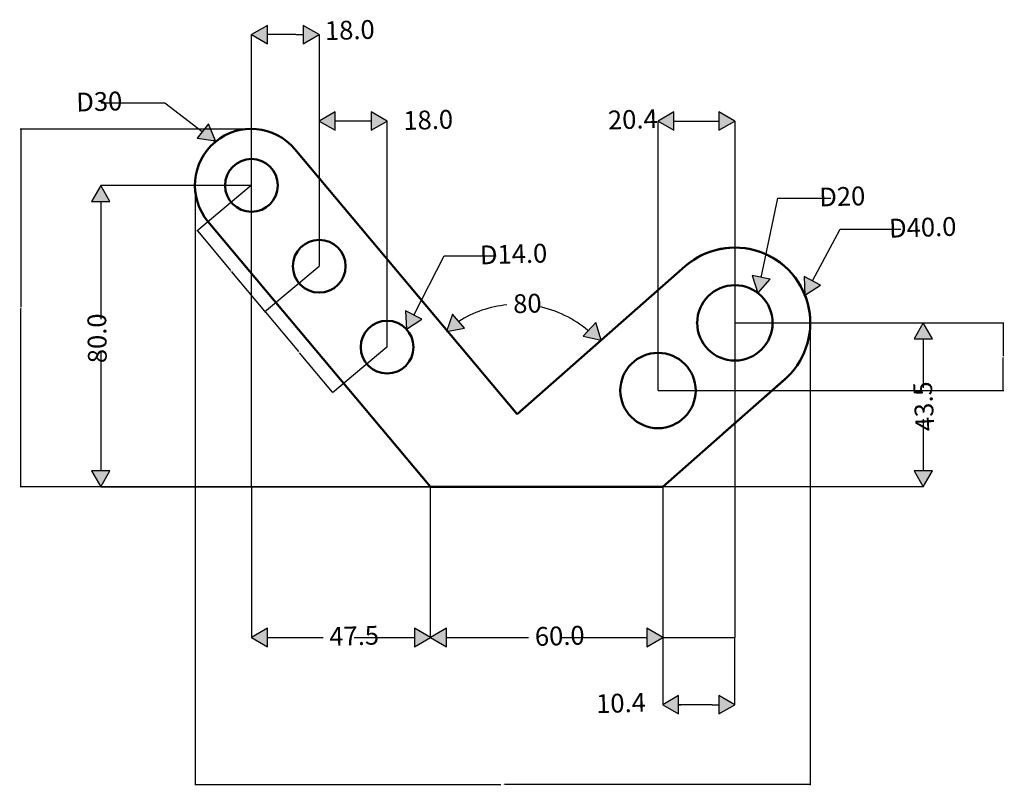
# Model space of a CAD drawing. Units: millimetres. Extents: x 651 to 912, y 1072 to 1275.
import ezdxf

# ---------------------------------------------------------------- set-up
doc = ezdxf.new("R2010")
doc.units = ezdxf.units.MM
for name, color, linetype, lineweight in [('M-CONS', 8, 'Continuous', 13), ('M-DIMS', 2, 'Continuous', 25), ('M-HATC', 2, 'Continuous', 18), ('M-OUTL', 7, 'Continuous', 50), ('M-TEXT', 7, 'Continuous', 25)]:
    doc.layers.add(name, color=color, linetype=linetype, lineweight=lineweight)
doc.styles.get("Standard").update_dxf_attribs({"font": 'arial.ttf'})
doc.dimstyles.get("Standard").update_dxf_attribs({"dimtxt": 0.18, "dimasz": 0.18, "dimexe": 0.18, "dimexo": 0.0625, "dimgap": 0.09, "dimtad": 0, "dimtih": 1, "dimtoh": 1, "dimdec": 4, "dimzin": 0, "dimdsep": 46, "dimtxsty": 'Standard', "dimcen": 0.09, "dimadec": 0, "dimazin": 0, "dimtfac": 1, "dimtdec": 4, "dimtofl": 0, "dimtmove": 0, "dimatfit": 3, "dimfxl": 1, "dimtolj": 1, "dimtzin": 0, "dimarcsym": 0})

# ---------------------------------------------------------------- blocks, each defined once
blk = doc.blocks.new('LINK-HOLE-D14')
blk.add_circle((7, 7), 7)
blk = doc.blocks.new('LINK-HOLE-D20')
blk.add_circle((10, 10), 10)
blk = doc.blocks.new('*D3')
at = {"layer": 'Defpoints', "color": 0, "transparency": 16777216}
for p in [(697.1, 1232.79), (860.34, 1194.98), (860.34, 1072.44)]:
    blk.add_point(p, dxfattribs=at)
at = {"layer": 'M-DIMS', "color": 0, "lineweight": -2, "transparency": 16777216}
for p, q in [((697.1, 1232.73), (697.1, 1072.26)), ((860.34, 1194.92), (860.34, 1072.26)), ((697.28, 1072.44), (778.26, 1072.44)), ((860.16, 1072.44), (779.17, 1072.44))]:
    blk.add_line(p, q, dxfattribs=at)
at = {"layer": 'M-DIMS', "color": 0, "transparency": 16777216}
for points in [[(697.28, 1072.47), (697.28, 1072.41), (697.1, 1072.44)], [(860.16, 1072.47), (860.16, 1072.41), (860.34, 1072.44)]]:
    blk.add_solid(points, dxfattribs=at)
at = {"layer": 'M-DIMS', "color": 0, "transparency": 16777216, "insert": (778.72, 1072.44), "char_height": 0.18, "attachment_point": 5}
blk.add_mtext('\\A1;163.24', dxfattribs=at)
blk = doc.blocks.new('*D4')
at = {"layer": 'Defpoints', "color": 0, "transparency": 16777216}
for p in [(713.35, 1246.42), (650.84, 1151.48), (759.54, 1151.48)]:
    blk.add_point(p, dxfattribs=at)
at = {"layer": 'M-DIMS', "color": 0, "lineweight": -2, "transparency": 16777216}
for p, q in [((713.29, 1246.42), (650.66, 1246.42)), ((650.84, 1246.24), (650.84, 1199.13)), ((650.84, 1151.66), (650.84, 1198.77)), ((759.48, 1151.48), (650.66, 1151.48))]:
    blk.add_line(p, q, dxfattribs=at)
at = {"layer": 'M-DIMS', "color": 0, "transparency": 16777216}
for points in [[(650.81, 1246.24), (650.87, 1246.24), (650.84, 1246.42)], [(650.81, 1151.66), (650.87, 1151.66), (650.84, 1151.48)]]:
    blk.add_solid(points, dxfattribs=at)
at = {"layer": 'M-DIMS', "color": 0, "transparency": 16777216, "insert": (650.84, 1198.95), "char_height": 0.18, "attachment_point": 5}
blk.add_mtext('\\A1;94.94', dxfattribs=at)
blk = doc.blocks.new('*D5')
at = {"layer": 'Defpoints', "color": 0, "transparency": 16777216}
for p in [(712.04, 1231.48), (697.67, 1219.43), (730.04, 1210.01)]:
    blk.add_point(p, dxfattribs=at)
at = {"layer": 'M-DIMS', "color": 0, "lineweight": -2, "transparency": 16777216}
for p, q in [((711.99, 1231.44), (697.53, 1219.32)), ((697.79, 1219.29), (706.52, 1208.88)), ((729.99, 1209.97), (715.53, 1197.85)), ((715.55, 1198.1), (706.82, 1208.52))]:
    blk.add_line(p, q, dxfattribs=at)
at = {"layer": 'M-DIMS', "color": 0, "transparency": 16777216}
for points in [[(697.81, 1219.31), (697.76, 1219.27), (697.67, 1219.43)], [(715.58, 1198.12), (715.53, 1198.08), (715.67, 1197.96)]]:
    blk.add_solid(points, dxfattribs=at)
at = {"layer": 'M-DIMS', "color": 0, "transparency": 16777216, "insert": (706.67, 1208.7), "char_height": 0.18, "attachment_point": 5}
blk.add_mtext('\\A1;28.016', dxfattribs=at)
blk = doc.blocks.new('*D6')
at = {"layer": 'Defpoints', "color": 0, "transparency": 16777216}
for p in [(730.04, 1210.01), (715.67, 1197.96), (748.04, 1188.54)]:
    blk.add_point(p, dxfattribs=at)
at = {"layer": 'M-DIMS', "color": 0, "lineweight": -2, "transparency": 16777216}
for p, q in [((729.99, 1209.97), (715.53, 1197.85)), ((715.79, 1197.82), (724.52, 1187.41)), ((733.55, 1176.63), (724.82, 1187.05)), ((747.99, 1188.5), (733.53, 1176.38))]:
    blk.add_line(p, q, dxfattribs=at)
at = {"layer": 'M-DIMS', "color": 0, "transparency": 16777216}
for points in [[(715.81, 1197.84), (715.76, 1197.81), (715.67, 1197.96)], [(733.58, 1176.65), (733.53, 1176.61), (733.67, 1176.49)]]:
    blk.add_solid(points, dxfattribs=at)
at = {"layer": 'M-DIMS', "color": 0, "transparency": 16777216, "insert": (724.67, 1187.23), "char_height": 0.18, "attachment_point": 5}
blk.add_mtext('\\A1;28.016', dxfattribs=at)
blk = doc.blocks.new('*D7')
at = {"layer": 'Defpoints', "color": 0, "transparency": 16777216}
for p in [(840.34, 1194.98), (911.54, 1194.98), (819.94, 1177.03)]:
    blk.add_point(p, dxfattribs=at)
at = {"layer": 'M-DIMS', "color": 0, "lineweight": -2, "transparency": 16777216}
for p, q in [((840.4, 1194.98), (911.72, 1194.98)), ((911.54, 1194.8), (911.54, 1186.19)), ((911.54, 1177.21), (911.54, 1185.82)), ((820, 1177.03), (911.72, 1177.03))]:
    blk.add_line(p, q, dxfattribs=at)
at = {"layer": 'M-DIMS', "color": 0, "transparency": 16777216}
for points in [[(911.51, 1194.8), (911.57, 1194.8), (911.54, 1194.98)], [(911.51, 1177.21), (911.57, 1177.21), (911.54, 1177.03)]]:
    blk.add_solid(points, dxfattribs=at)
at = {"layer": 'M-DIMS', "color": 0, "transparency": 16777216, "insert": (911.54, 1186), "char_height": 0.18, "attachment_point": 5}
blk.add_mtext('\\A1;17.95', dxfattribs=at)

msp = doc.modelspace()

# ---------------------------------------------------------------- hatches: boundary and pattern name
at = {"layer": 'M-HATC'}
h = msp.add_hatch(color=256, dxfattribs=at)
h.dxf.hatch_style = 1
h.paths.add_polyline_path([(700.674, 1247.8423), (697.6175, 1244.0165), (702.459, 1243.2824)])
h.paths.add_polyline_path([(672.0381, 1231.4781), (669.5896, 1227.2373), (674.4865, 1227.2373)])
h.paths.add_polyline_path([(674.4865, 1155.7189), (669.5896, 1155.7189), (672.0381, 1151.4781)])
h.paths.add_polyline_path([(716.2789, 1273.9265), (712.0381, 1271.4781), (716.2789, 1269.0297)])
h.paths.add_polyline_path([(725.7973, 1273.9265), (725.7973, 1269.0297), (730.0381, 1271.4781)])
h.paths.add_polyline_path([(734.2789, 1250.9893), (730.0381, 1248.5409), (734.2789, 1246.0925)])
h.paths.add_polyline_path([(748.0381, 1248.5409), (743.7973, 1250.9893), (743.7973, 1246.0925)])
h.paths.add_polyline_path([(757.2809, 1195.9676), (752.9115, 1198.1782), (753.1818, 1193.2888)])
h.paths.add_polyline_path([(768.5844, 1193.5434), (765.4383, 1197.2959), (763.8732, 1193.0011), (764.0825, 1192.7514)])
h.paths.add_polyline_path([(824.1789, 1250.9893), (819.9381, 1248.5409), (824.1789, 1246.0925)])
h.paths.add_polyline_path([(836.0973, 1250.9893), (836.0973, 1246.0925), (840.3381, 1248.5409)])
h.paths.add_polyline_path([(849.6943, 1206.5585), (844.901, 1207.5604), (846.4299, 1202.9084)])
h.paths.add_polyline_path([(863.0836, 1204.9487), (858.766, 1207.259), (858.924, 1202.3647)])
h.paths.add_polyline_path([(890.3381, 1194.9781), (887.8896, 1190.7373), (892.7865, 1190.7373)])
h.paths.add_polyline_path([(892.7865, 1155.7189), (887.8896, 1155.7189), (890.3381, 1151.4781)])
h.paths.add_polyline_path([(836.0973, 1096.0877), (836.0973, 1091.1908), (840.3381, 1093.6392)])
h.paths.add_polyline_path([(825.4154, 1096.0877), (821.1746, 1093.6392), (825.4154, 1091.1908)])
h.paths.add_polyline_path([(821.1746, 1111.4781), (816.9338, 1113.9265), (816.9338, 1109.0297)])
h.paths.add_polyline_path([(763.7789, 1113.9265), (759.5381, 1111.4781), (763.7789, 1109.0297)])
h.paths.add_polyline_path([(759.5381, 1111.4781), (755.2973, 1113.9265), (755.2973, 1109.0297)])
h.paths.add_polyline_path([(716.2789, 1113.9265), (712.0381, 1111.4781), (716.2789, 1109.0297)])
h = msp.add_hatch(color=256, dxfattribs=at)
h.dxf.hatch_style = 1
h.paths.add_polyline_path([(803.4019, 1195.0581), (800.0571, 1191.4816), (804.8269, 1190.3732)])

# ---------------------------------------------------------------- linework, layer by layer
at = {"layer": 'M-CONS'}
for p, q in [((712.0381, 1151.4781), (712.0381, 1208.1314)), ((829.9381, 1194.9781), (830.3381, 1194.9781))]:
    msp.add_line(p, q, dxfattribs=at)
at = {"layer": 'M-DIMS'}
for p, q in [((712.0381, 1231.4781), (712.0381, 1271.4781)), ((723.8412, 1271.4781), (716.2789, 1271.4781)), ((723.8412, 1271.4781), (725.7973, 1271.4781)), ((730.0381, 1271.4781), (730.0381, 1210.0095)), ((689.0673, 1253.2901), (672.1881, 1253.2901)), ((698.9295, 1245.6587), (689.0673, 1253.2901)), ((734.2854, 1248.5409), (734.2789, 1248.5409)), ((742.5886, 1248.5409), (734.2854, 1248.5409)), ((743.7973, 1248.5409), (742.5886, 1248.5409)), ((748.0381, 1188.5409), (748.0381, 1248.5409)), ((819.9381, 1177.0294), (819.9381, 1248.5409)), ((824.1789, 1248.5409), (836.0973, 1248.5409)), ((840.3381, 1248.5409), (840.3381, 1194.9781)), ((702.4008, 1242.9725), (701.8886, 1243.3689)), ((712.0381, 1231.4781), (672.0381, 1231.4781)), ((712.0381, 1151.4781), (712.0381, 1231.4781)), ((672.0381, 1227.2373), (672.0381, 1195.9725)), ((847.2976, 1207.0595), (851.6967, 1228.1047)), ((851.6967, 1228.1047), (865.831, 1228.1047)), ((860.9248, 1206.1039), (868.2679, 1219.8272)), ((868.2679, 1219.8272), (884.3518, 1219.8272)), ((755.1235, 1197.0591), (763.1997, 1212.7406)), ((763.1997, 1212.7406), (776.9484, 1212.7406)), ((840.3381, 1194.9781), (890.3381, 1194.9781)), ((840.3381, 1194.9781), (840.3381, 1111.4781)), ((890.3381, 1190.7373), (890.3381, 1177.7225)), ((672.0381, 1187.6489), (672.0381, 1155.7189)), ((890.3381, 1169.3989), (890.3381, 1155.7189)), ((672.0381, 1151.4781), (712.0381, 1151.4781)), ((712.0381, 1151.4781), (759.5381, 1151.4781)), ((712.0381, 1151.4781), (712.0381, 1111.4781)), ((759.5381, 1111.4781), (759.5381, 1151.4781)), ((890.3381, 1151.4781), (821.1746, 1151.4781)), ((821.1746, 1151.4781), (821.1746, 1111.4781)), ((716.2789, 1111.4781), (731.0354, 1111.4781)), ((739.3386, 1111.4781), (755.2973, 1111.4781)), ((763.7789, 1111.4781), (785.6037, 1111.4781)), ((793.9069, 1111.4781), (816.9338, 1111.4781)), ((821.1746, 1111.4781), (821.1746, 1093.6392)), ((821.1746, 1111.4781), (826.71, 1111.4781)), ((826.71, 1111.4781), (840.3381, 1111.4781)), ((840.3381, 1093.6392), (840.3381, 1111.4781)), ((825.4154, 1093.6392), (826.0037, 1093.6392)), ((834.3069, 1093.6392), (825.4154, 1093.6392)), ((834.3069, 1093.6392), (836.0973, 1093.6392))]:
    msp.add_line(p, q, dxfattribs=at)
for points in [[(712.0381, 1271.4781), (716.2789, 1269.0297), (716.2789, 1273.9265)], [(730.0381, 1271.4781), (725.7973, 1273.9265), (725.7973, 1269.0297)], [(730.0381, 1248.5409), (734.2789, 1246.0925), (734.2789, 1250.9893)], [(748.0381, 1248.5409), (743.7973, 1250.9893), (743.7973, 1246.0925)], [(819.9381, 1248.5409), (824.1789, 1246.0925), (824.1789, 1250.9893)], [(840.3381, 1248.5409), (836.0973, 1250.9893), (836.0973, 1246.0925)], [(702.459, 1243.2824), (700.674, 1247.8423), (697.6175, 1244.0165)], [(672.0381, 1231.4781), (669.5896, 1227.2373), (674.4865, 1227.2373)], [(846.4299, 1202.9084), (849.6943, 1206.5585), (844.901, 1207.5604)], [(858.924, 1202.3647), (863.0836, 1204.9487), (858.766, 1207.259)], [(753.1818, 1193.2888), (757.2809, 1195.9676), (752.9115, 1198.1782)], [(763.7616, 1192.695), (768.5844, 1193.5434), (765.4383, 1197.2959)], [(804.8269, 1190.3732), (803.4019, 1195.0581), (800.0571, 1191.4816)], [(890.3381, 1194.9781), (887.8896, 1190.7373), (892.7865, 1190.7373)], [(672.0381, 1151.4781), (674.4865, 1155.7189), (669.5896, 1155.7189)], [(890.3381, 1151.4781), (892.7865, 1155.7189), (887.8896, 1155.7189)], [(712.0381, 1111.4781), (716.2789, 1109.0297), (716.2789, 1113.9265)], [(759.5381, 1111.4781), (755.2973, 1113.9265), (755.2973, 1109.0297)], [(759.5381, 1111.4781), (763.7789, 1109.0297), (763.7789, 1113.9265)], [(821.1746, 1111.4781), (816.9338, 1113.9265), (816.9338, 1109.0297)], [(821.1746, 1093.6392), (825.4154, 1091.1908), (825.4154, 1096.0877)], [(840.3381, 1093.6392), (836.0973, 1096.0877), (836.0973, 1091.1908)]]:
    msp.add_lwpolyline(points, close=True, dxfattribs=at)
for start, end in [(95.296054, 122.160224), (49.703655, 78.846753), (129.73754, 129.9776), (41.34262587546275, 41.34262629260944)]:
    msp.add_arc((782.5269, 1170.7527), 29.1043, start, end, dxfattribs=at)
at = {"layer": 'M-OUTL'}
for p, q in [((782.5269, 1170.7527), (723.5325, 1241.1154)), ((759.5381, 1151.4781), (700.5436, 1221.8408)), ((782.5269, 1170.7527), (827.1269, 1209.9936)), ((821.1746, 1151.4781), (853.5493, 1179.9626)), ((837.3619, 1165.7204), (853.7671, 1180.1572)), ((759.5381, 1151.4781), (819.5381, 1151.4781)), ((819.5381, 1151.4781), (821.1746, 1151.4781)), ((821.1746, 1151.4781), (819.5381, 1151.4781))]:
    msp.add_line(p, q, dxfattribs=at)
for centre, radius, start, end in [((712.0381, 1231.4781), 15, 39.9776, 219.9776), ((840.3381, 1194.9781), 20, 0, 131.342626), ((840.3381, 1194.9781), 20, 310.517125, 131.342626)]:
    msp.add_arc(centre, radius, start, end, dxfattribs=at)

# ---------------------------------------------------------------- block references
for name, p in [('LINK-HOLE-D14', (705.038, 1224.478)), ('LINK-HOLE-D14', (723.038, 1203.0094)), ('LINK-HOLE-D20', (830.338, 1184.978)), ('LINK-HOLE-D14', (741.038, 1181.5408)), ('LINK-HOLE-D20', (809.938, 1167.0293))]:
    msp.add_blockref(name, p, dxfattribs=at)

# ---------------------------------------------------------------- texts
at = {"layer": 'M-TEXT', "char_height": 4.97962, "attachment_point": 1}
for s, insert, rotation in [('18.0', (731.464, 1274.9854), 1.741586), ('D30', (665.4623, 1256.0273), 1.741586), ('18.0', (752.2708, 1251.1404), 1.741586), ('20.4', (806.5765, 1251.2781), 1.741586), ('D20', (862.6558, 1230.8419), 1.741586), ('D40.0', (881.1766, 1222.5644), 1.741586), ('D14.0', (772.5843, 1215.4778), 1.741586), ('80', (781.4164, 1202.5209), 1.741586), ('80.0', (668.6739, 1184.2423), 90.76983), ('43.5', (888.3412, 1166.0909), 93.156428), ('47.5', (732.6129, 1114.2153), 1.741586), ('60.0', (787.1811, 1114.2153), 1.741586), ('10.4', (803.4367, 1096.3765), 1.741586)]:
    msp.add_mtext_dynamic_manual_height_columns(s, width=4.97962, gutter_width=24.8981, heights=[0], dxfattribs=dict(at, insert=insert, rotation=rotation))

# ---------------------------------------------------------------- dimensions: what is measured, and where the dimension line sits
at = {"layer": 'M-DIMS'}
for base, p1, p2, angle, override, picture, middle in [((650.8396, 1151.4781), (713.3513, 1246.4205), (759.5381, 1151.4781), 90, {"dimdec": 2, "dimlfac": 1, "dimrnd": 0, "dimzin": 0, "dimdsep": 46, "dimlunit": 2}, '*D4', (650.8396, 1198.9493)), ((697.67, 1219.4315), (730.0381, 1210.0095), (712.0381, 1231.4781), 129.9776, {"dimdec": 3, "dimlfac": 1, "dimrnd": 0, "dimzin": 0, "dimdsep": 46, "dimlunit": 2}, '*D5', (706.67, 1208.6972)), ((715.67, 1197.9629), (748.0381, 1188.5409), (730.0381, 1210.0095), 129.9776, {"dimdec": 3, "dimlfac": 1, "dimrnd": 0, "dimzin": 0, "dimdsep": 46, "dimlunit": 2}, '*D6', (724.67, 1187.2285)), ((911.5365, 1194.9781), (819.9381, 1177.0294), (840.3381, 1194.9781), 90, {"dimdec": 2, "dimlfac": 1, "dimrnd": 0, "dimzin": 0, "dimdsep": 46, "dimlunit": 2}, '*D7', (911.5365, 1186.0037))]:
    dim = msp.add_linear_dim(base=base, p1=p1, p2=p2, angle=angle, dimstyle='Standard', override=override, dxfattribs=at)
    dim.commit()
    dim.dimension.update_dxf_attribs({"geometry": picture, "text_midpoint": middle})
dim = msp.add_linear_dim(base=(860.3381, 1072.4408), p1=(697.0957, 1232.7913), p2=(860.3381, 1194.9781), dimstyle='Standard', override={"dimdec": 2, "dimlfac": 1, "dimrnd": 0, "dimzin": 0, "dimdsep": 46, "dimlunit": 2}, dxfattribs=at)
dim.commit()
dim.dimension.update_dxf_attribs({"geometry": '*D3', "text_midpoint": (778.7169, 1072.4408)})

doc.saveas('drawing.dxf')
